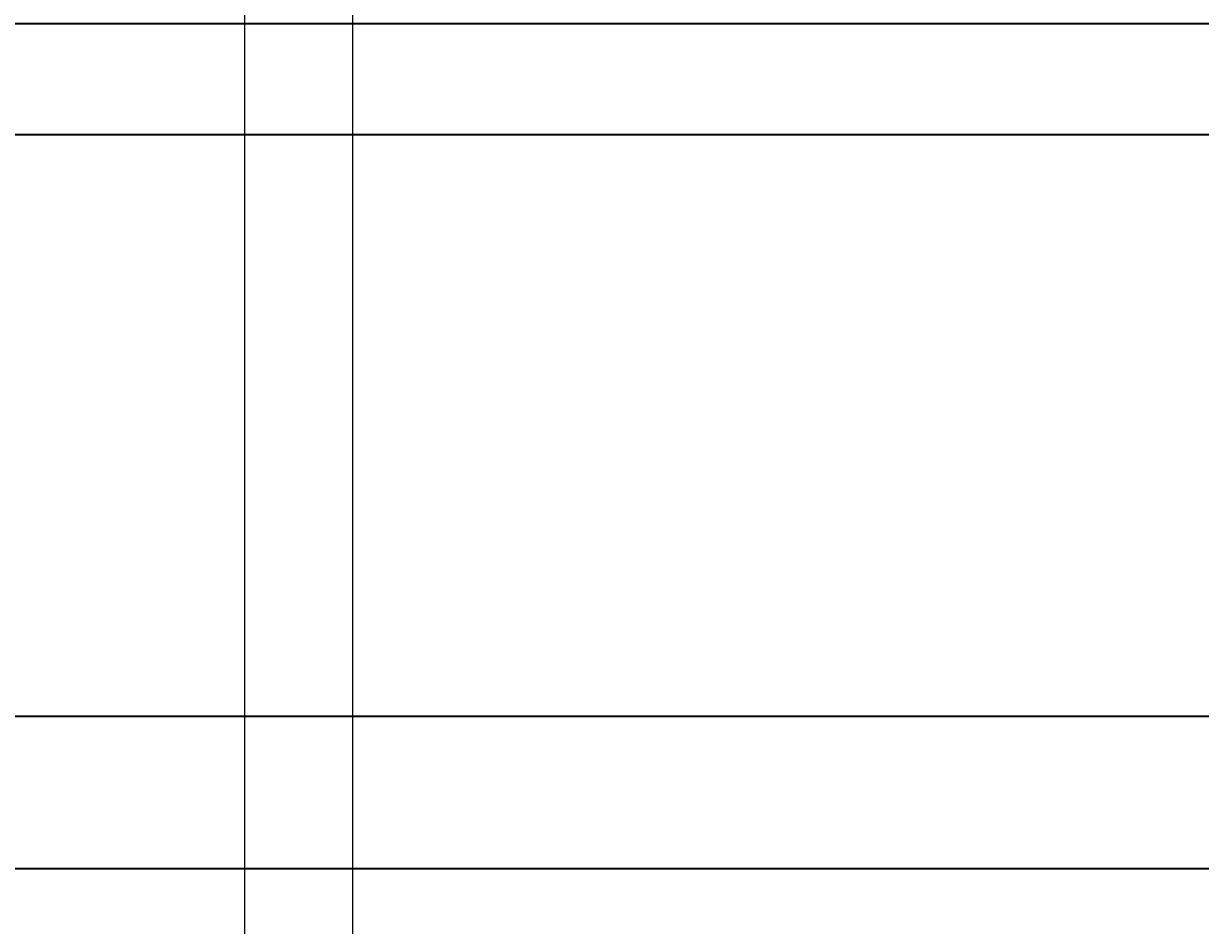
# Model space of a CAD drawing. Units: inches. Extents: x -6 to 289, y -8 to 323.
# Tile 100 of 107: x 196 to 219, y 276 to 294. Entities that reach past the tile are written whole.
import ezdxf

# ---------------------------------------------------------------- set-up
doc = ezdxf.new("R2010")
doc.units = ezdxf.units.IN
doc.header["$MEASUREMENT"] = 0
doc.layers.add('A-ANNO-DIMS', color=2, linetype='Continuous', lineweight=18)
doc.layers.add('A-ELEV', color=7, linetype='Continuous', lineweight=35)
doc.styles.get("Standard").update_dxf_attribs({"font": 'arial.ttf'})
doc.dimstyles.get("Standard").update_dxf_attribs({"dimtxt": 0.18, "dimasz": 0.18, "dimexe": 0.18, "dimexo": 0.0625, "dimgap": 0.09, "dimtad": 0, "dimtih": 1, "dimtoh": 1, "dimdec": 4, "dimzin": 0, "dimdsep": 46, "dimtxsty": 'Standard', "dimcen": 0.09, "dimadec": 0, "dimazin": 0, "dimtfac": 1, "dimtdec": 4, "dimtofl": 0, "dimtmove": 0, "dimatfit": 3, "dimfxl": 1, "dimtolj": 1, "dimtzin": 0, "dimarcsym": 0})

# ---------------------------------------------------------------- blocks, each defined once
blk = doc.blocks.new('*D13')
at = {"layer": 'A-ANNO-DIMS', "color": 0, "lineweight": -2, "transparency": 16777216}
for p, q in [((188.292, 226.951), (188.292, 322.969)), ((236.292, 226.951), (236.292, 322.969)), ((188.472, 322.789), (212.069, 322.789)), ((236.112, 322.789), (212.515, 322.789))]:
    blk.add_line(p, q, dxfattribs=at)
at = {"layer": 'A-ANNO-DIMS', "color": 0, "transparency": 16777216}
for points in [[(188.472, 322.819), (188.472, 322.759), (188.292, 322.789)], [(236.112, 322.819), (236.112, 322.759), (236.292, 322.789)]]:
    blk.add_solid(points, dxfattribs=at)
at = {"layer": 'Defpoints', "color": 0, "transparency": 16777216}
for p in [(236.292, 322.789), (188.292, 226.889), (236.292, 226.889)]:
    blk.add_point(p, dxfattribs=at)
at = {"layer": 'A-ANNO-DIMS', "color": 0, "transparency": 16777216, "insert": (212.292, 322.789), "char_height": 0.18, "attachment_point": 5}
blk.add_mtext('\\A1;48', dxfattribs=at)
blk = doc.blocks.new('*D27')
at = {"layer": 'A-ANNO-DIMS', "color": 0, "lineweight": -2, "transparency": 16777216}
for p, q in [((19.226, 307.289), (288.653, 307.289)), ((288.473, 307.109), (288.473, 277.471)), ((288.473, 247.469), (288.473, 277.107)), ((247.226, 247.289), (288.653, 247.289))]:
    blk.add_line(p, q, dxfattribs=at)
at = {"layer": 'A-ANNO-DIMS', "color": 0, "transparency": 16777216}
for points in [[(288.443, 307.109), (288.503, 307.109), (288.473, 307.289)], [(288.443, 247.469), (288.503, 247.469), (288.473, 247.289)]]:
    blk.add_solid(points, dxfattribs=at)
at = {"layer": 'Defpoints', "color": 0, "transparency": 16777216}
for p in [(19.164, 307.289), (288.473, 307.289), (247.164, 247.289)]:
    blk.add_point(p, dxfattribs=at)
at = {"layer": 'A-ANNO-DIMS', "color": 0, "transparency": 16777216, "insert": (288.473, 277.289), "char_height": 0.18, "attachment_point": 5}
blk.add_mtext('\\A1;60', dxfattribs=at)
blk = doc.blocks.new('*D80')
at = {"layer": 'A-ANNO-DIMS', "color": 0, "lineweight": -2, "transparency": 16777216}
for p, q in [((188.292, 116.842), (188.292, 322.969)), ((230.292, 116.842), (230.292, 322.969)), ((188.472, 322.789), (209.07, 322.789)), ((230.112, 322.789), (209.513, 322.789))]:
    blk.add_line(p, q, dxfattribs=at)
at = {"layer": 'A-ANNO-DIMS', "color": 0, "transparency": 16777216}
for points in [[(188.472, 322.819), (188.472, 322.759), (188.292, 322.789)], [(230.112, 322.819), (230.112, 322.759), (230.292, 322.789)]]:
    blk.add_solid(points, dxfattribs=at)
at = {"layer": 'Defpoints', "color": 0, "transparency": 16777216}
for p in [(230.292, 322.789), (188.292, 116.779), (230.292, 116.779)]:
    blk.add_point(p, dxfattribs=at)
at = {"layer": 'A-ANNO-DIMS', "color": 0, "transparency": 16777216, "insert": (209.292, 322.789), "char_height": 0.18, "attachment_point": 5}
blk.add_mtext('\\A1;42', dxfattribs=at)
blk = doc.blocks.new('*D96')
at = {"layer": 'A-ANNO-DIMS', "color": 0, "lineweight": -2, "transparency": 16777216}
for p, q in [((164.004, 159.411), (164.004, 322.969)), ((200.616, 159.411), (200.616, 322.969)), ((164.184, 322.789), (181.934, 322.789)), ((200.436, 322.789), (182.686, 322.789))]:
    blk.add_line(p, q, dxfattribs=at)
at = {"layer": 'A-ANNO-DIMS', "color": 0, "transparency": 16777216}
for points in [[(164.184, 322.819), (164.184, 322.759), (164.004, 322.789)], [(200.436, 322.819), (200.436, 322.759), (200.616, 322.789)]]:
    blk.add_solid(points, dxfattribs=at)
at = {"layer": 'Defpoints', "color": 0, "transparency": 16777216}
for p in [(200.616, 322.789), (164.004, 159.348), (200.616, 159.348)]:
    blk.add_point(p, dxfattribs=at)
at = {"layer": 'A-ANNO-DIMS', "color": 0, "transparency": 16777216, "insert": (182.31, 322.789), "char_height": 0.18, "attachment_point": 5}
blk.add_mtext('\\A1;36.61', dxfattribs=at)
blk = doc.blocks.new('*D97')
at = {"layer": 'A-ANNO-DIMS', "color": 0, "lineweight": -2, "transparency": 16777216}
for p, q in [((200.616, 159.411), (200.616, 322.969)), ((202.741, 159.411), (202.741, 322.969)), ((200.796, 322.789), (201.283, 322.789)), ((202.561, 322.789), (202.075, 322.789))]:
    blk.add_line(p, q, dxfattribs=at)
at = {"layer": 'A-ANNO-DIMS', "color": 0, "transparency": 16777216}
for points in [[(200.796, 322.819), (200.796, 322.759), (200.616, 322.789)], [(202.561, 322.819), (202.561, 322.759), (202.741, 322.789)]]:
    blk.add_solid(points, dxfattribs=at)
at = {"layer": 'Defpoints', "color": 0, "transparency": 16777216}
for p in [(202.741, 322.789), (200.616, 159.348), (202.741, 159.348)]:
    blk.add_point(p, dxfattribs=at)
at = {"layer": 'A-ANNO-DIMS', "color": 0, "transparency": 16777216, "insert": (201.679, 322.789), "char_height": 0.18, "attachment_point": 5}
blk.add_mtext('\\A1;2.125', dxfattribs=at)
blk = doc.blocks.new('*D98')
at = {"layer": 'A-ANNO-DIMS', "color": 0, "lineweight": -2, "transparency": 16777216}
for p, q in [((202.741, 159.411), (202.741, 322.969)), ((244.164, 159.411), (244.164, 322.969)), ((202.921, 322.789), (223.056, 322.789)), ((243.984, 322.789), (223.849, 322.789))]:
    blk.add_line(p, q, dxfattribs=at)
at = {"layer": 'A-ANNO-DIMS', "color": 0, "transparency": 16777216}
for points in [[(202.921, 322.819), (202.921, 322.759), (202.741, 322.789)], [(243.984, 322.819), (243.984, 322.759), (244.164, 322.789)]]:
    blk.add_solid(points, dxfattribs=at)
at = {"layer": 'Defpoints', "color": 0, "transparency": 16777216}
for p in [(244.164, 322.789), (202.741, 159.348), (244.164, 159.348)]:
    blk.add_point(p, dxfattribs=at)
at = {"layer": 'A-ANNO-DIMS', "color": 0, "transparency": 16777216, "insert": (223.452, 322.789), "char_height": 0.18, "attachment_point": 5}
blk.add_mtext('\\A1;41.42', dxfattribs=at)
blk = doc.blocks.new('*D108')
at = {"layer": 'A-ANNO-DIMS', "color": 0, "lineweight": -2, "transparency": 16777216}
for p, q in [((186.984, 291.541), (186.984, 322.969)), ((255.804, 291.541), (255.804, 322.969)), ((187.164, 322.789), (221, 322.789)), ((255.624, 322.789), (221.787, 322.789))]:
    blk.add_line(p, q, dxfattribs=at)
at = {"layer": 'A-ANNO-DIMS', "color": 0, "transparency": 16777216}
for points in [[(187.164, 322.819), (187.164, 322.759), (186.984, 322.789)], [(255.624, 322.819), (255.624, 322.759), (255.804, 322.789)]]:
    blk.add_solid(points, dxfattribs=at)
at = {"layer": 'Defpoints', "color": 0, "transparency": 16777216}
for p in [(255.804, 322.789), (186.984, 291.478), (255.804, 291.478)]:
    blk.add_point(p, dxfattribs=at)
at = {"layer": 'A-ANNO-DIMS', "color": 0, "transparency": 16777216, "insert": (221.394, 322.789), "char_height": 0.18, "attachment_point": 5}
blk.add_mtext('\\A1;68.82', dxfattribs=at)

msp = doc.modelspace()

# ---------------------------------------------------------------- linework, layer by layer
at = {"layer": 'A-ELEV'}
for points in [[(115.1638, 307.2888), (115.1638, 277.0427), (259.1638, 277.0427), (259.1638, 259.2888)], [(118.1638, 307.2888), (118.1638, 280.0427), (262.1638, 280.0427), (262.1638, 259.2888)], [(255.8036, 291.4781), (118.1638, 291.4781), (118.1638, 293.6657), (255.8036, 293.6657)]]:
    msp.add_lwpolyline(points, dxfattribs=at)

# ---------------------------------------------------------------- dimensions: what is measured, and where the dimension line sits
at = {"layer": 'A-ANNO-DIMS'}
for base, p1, p2, override, picture, middle in [((200.6162, 322.7888), (164.0039, 159.3484), (200.6162, 159.3484), {"dimdec": 2, "dimlfac": 1, "dimrnd": 0, "dimzin": 0, "dimdsep": 46, "dimlunit": 2}, '*D96', (182.3101, 322.7888)), ((255.8036, 322.7888), (186.9837, 291.4781), (255.8036, 291.4781), {"dimdec": 2, "dimlfac": 1, "dimrnd": 0, "dimzin": 0, "dimdsep": 46, "dimlunit": 2}, '*D108', (221.3936, 322.7888)), ((236.2918, 322.7888), (188.2918, 226.8887), (236.2918, 226.8887), {"dimdec": 0, "dimlfac": 1, "dimrnd": 0, "dimzin": 0, "dimdsep": 46, "dimlunit": 2}, '*D13', (212.2918, 322.7888)), ((230.2918, 322.7888), (188.2918, 116.7795), (230.2918, 116.7795), {"dimdec": 0, "dimlfac": 1, "dimrnd": 0, "dimzin": 0, "dimdsep": 46, "dimlunit": 2}, '*D80', (209.2918, 322.7888)), ((202.741, 322.7888), (200.6162, 159.3484), (202.741, 159.3484), {"dimdec": 3, "dimlfac": 1, "dimrnd": 0, "dimzin": 0, "dimdsep": 46, "dimlunit": 2}, '*D97', (201.6786, 322.7888)), ((244.1638, 322.7888), (202.741, 159.3484), (244.1638, 159.3484), {"dimdec": 2, "dimlfac": 1, "dimrnd": 0, "dimzin": 0, "dimdsep": 46, "dimlunit": 2}, '*D98', (223.4524, 322.7888))]:
    dim = msp.add_linear_dim(base=base, p1=p1, p2=p2, dimstyle='Standard', override=override, dxfattribs=at)
    dim.commit()
    dim.dimension.update_dxf_attribs({"geometry": picture, "text_midpoint": middle})
dim = msp.add_linear_dim(base=(288.4733, 307.2888), p1=(247.1638, 247.2888), p2=(19.1638, 307.2888), angle=90, dimstyle='Standard', override={"dimdec": 0, "dimlfac": 1, "dimrnd": 0, "dimzin": 0, "dimdsep": 46, "dimlunit": 2}, dxfattribs=at)
dim.commit()
dim.dimension.update_dxf_attribs({"geometry": '*D27', "text_midpoint": (288.4733, 277.2888)})

doc.saveas('drawing.dxf')
